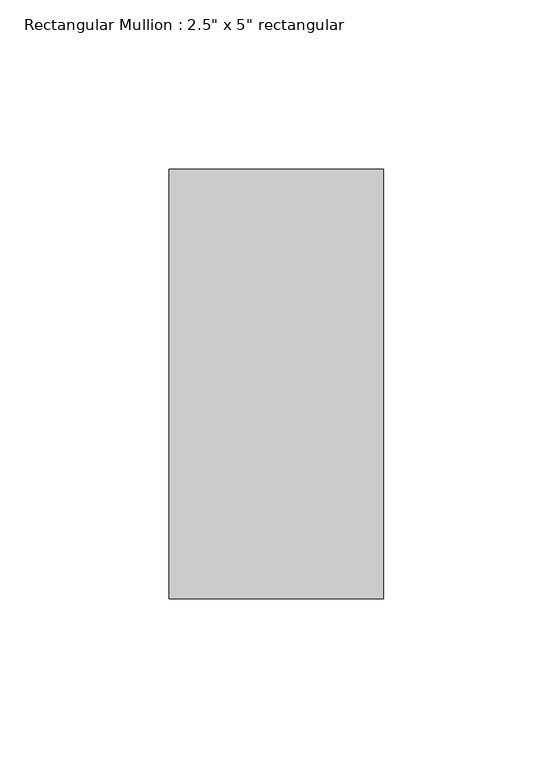
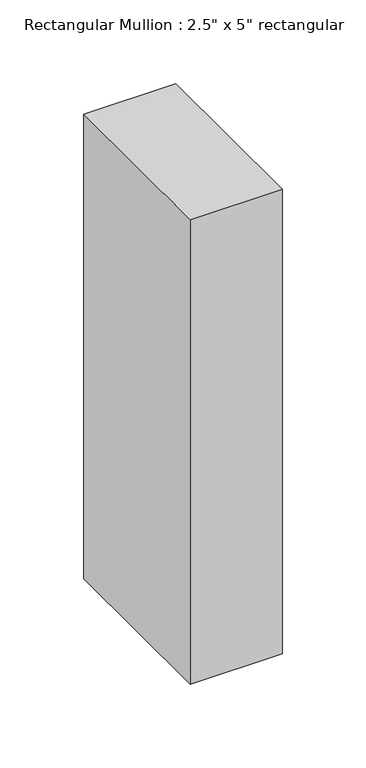
"""IFC4 building model written with IfcOpenShell, lengths in millimetres: member geometry."""

from ifc_helpers import new_model, si_unit, frame, origin, place, context, project, spatial, polyline, outline, extrude, source, transform, mapped, element, save


def member_fb4dac25(model_context):
    return source(origin(), model_context, "Body", "SweptSolid", [
        extrude(outline(polyline([(0.0, 63.5), (0.0, -63.5), (-63.5, -63.5), (-63.5, 63.5), (0.0, 63.5)])), frame((0.0, 0.0, -338.6666667), z_axis=(0.0, 0.0, 1.0), x_axis=(1.0, 0.0, 0.0)), (0.0, 0.0, 1.0), 338.6666667),
    ])


if __name__ == "__main__":
    model = new_model("IFC4")
    model_context = context("Model", 3, world=origin())
    ifc_project = project(units=[si_unit("LENGTHUNIT", "METRE", prefix="MILLI")], contexts=[model_context])
    site = spatial("IfcSite", under=ifc_project)
    building = spatial("IfcBuilding", under=site)
    placement = place(None, origin())
    member_shape = member_fb4dac25(model_context)
    element("IfcMember", 1, ObjectType="Rectangular Mullion : 2.5\" x 5\" rectangular", at=placement, inside=building, context=model_context, shape_type="MappedRepresentation", body=[
        mapped(member_shape, transform((0.0, 0.0, 0.0), x_axis=(1.0, 0.0, 0.0), y_axis=(0.0, 1.0, 0.0), z_axis=(0.0, 0.0, 1.0))),
    ])
    save(model, "model.ifc")

# Revit data of these elements
# Type "Rectangular Mullion : 2.5\" x 5\" rectangular"
#   built-in parameter 1007304 = 0.416667 (stored number, unit not read)
#   built-in parameter 1007301 = 0.104167 (stored number, unit not read)
#   built-in parameter 1007300 = 0.104167 (stored number, unit not read)
# Element 1 (IfcMember, "Rectangular Mullion : 2.5\" x 5\" rectangular")
#   Materials on its faces: "door colour"
# Materials
#   "door colour": class "Generic", colour RGB 120 120 120, transparency 0, Cost = 0
